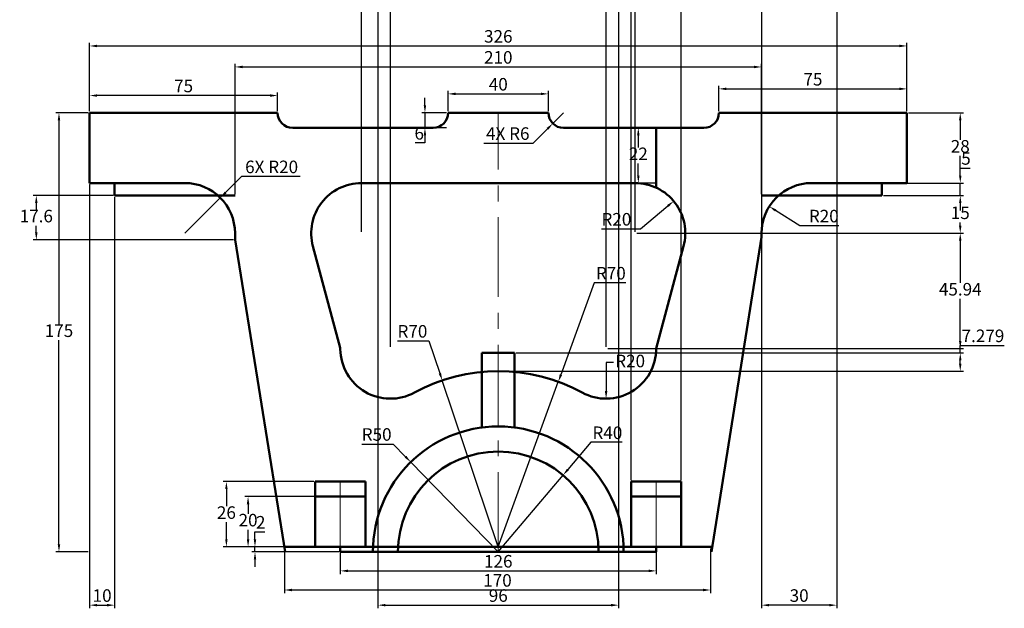
# Model space of a CAD drawing. Units: millimetres. Extents: x -44 to 350, y 28 to 429.
# Tile 1 of 2: x -43 to 350, y 28 to 262. Entities that reach past the tile are written whole.
import ezdxf

# ---------------------------------------------------------------- set-up
doc = ezdxf.new("R2010")
doc.units = ezdxf.units.MM
doc.linetypes.add('CENTER', pattern=[50.8, 31.75, -6.35, 6.35, -6.35])
for name, color, linetype, lineweight in [('M-CNTR', 1, 'CENTER', 18), ('M-DIMS', 2, 'Continuous', 25), ('M-OUTL', 7, 'Continuous', 50)]:
    doc.layers.add(name, color=color, linetype=linetype, lineweight=lineweight)
doc.styles.get("Standard").update_dxf_attribs({"font": 'arial.ttf'})
doc.dimstyles.new('ISO-25', dxfattribs={"dimtxt": 5, "dimasz": 3, "dimexe": 1.25, "dimexo": 0.625, "dimtad": 1, "dimtih": 1, "dimtoh": 1, "dimtxsty": 'Standard', "dimcen": 2.5, "dimadec": 0, "dimazin": 0, "dimtfac": 1, "dimtmove": 0, "dimatfit": 3, "dimfxl": 1, "dimarcsym": 0})

# ---------------------------------------------------------------- blocks, each defined once
blk = doc.blocks.new('*D1')
at = {"layer": 'Defpoints', "color": 0, "transparency": 16777216}
for p in [(310.7, 234.71), (235.7, 225.16), (310.7, 225.16)]:
    blk.add_point(p, dxfattribs=at)
at = {"layer": 'M-DIMS', "color": 0, "lineweight": -2, "transparency": 16777216}
for p, q in [((235.7, 225.78), (235.7, 235.96)), ((310.7, 225.78), (310.7, 235.96)), ((238.7, 234.71), (307.7, 234.71))]:
    blk.add_line(p, q, dxfattribs=at)
at = {"layer": 'M-DIMS', "color": 0, "transparency": 16777216}
for points in [[(238.7, 235.21), (238.7, 234.21), (235.7, 234.71)], [(307.7, 235.21), (307.7, 234.21), (310.7, 234.71)]]:
    blk.add_solid(points, dxfattribs=at)
at = {"layer": 'M-DIMS', "color": 0, "transparency": 16777216, "insert": (273.2, 237.88), "char_height": 5, "attachment_point": 5}
blk.add_mtext('75', dxfattribs=at)
blk = doc.blocks.new('*D2')
at = {"layer": 'Defpoints', "color": 0, "transparency": 16777216}
for p in [(167.7, 232.71), (127.7, 225.16), (167.7, 225.16)]:
    blk.add_point(p, dxfattribs=at)
at = {"layer": 'M-DIMS', "color": 0, "lineweight": -2, "transparency": 16777216}
for p, q in [((127.7, 225.78), (127.7, 233.96)), ((130.7, 232.71), (164.7, 232.71)), ((167.7, 225.78), (167.7, 233.96))]:
    blk.add_line(p, q, dxfattribs=at)
at = {"layer": 'M-DIMS', "color": 0, "transparency": 16777216}
for points in [[(130.7, 233.21), (130.7, 232.21), (127.7, 232.71)], [(164.7, 233.21), (164.7, 232.21), (167.7, 232.71)]]:
    blk.add_solid(points, dxfattribs=at)
at = {"layer": 'M-DIMS', "color": 0, "transparency": 16777216, "insert": (147.7, 235.89), "char_height": 5, "attachment_point": 5}
blk.add_mtext('40', dxfattribs=at)
blk = doc.blocks.new('*D3')
at = {"layer": 'Defpoints', "color": 0, "transparency": 16777216}
for p in [(-15.3, 232.04), (-15.3, 225.16), (59.7, 225.16)]:
    blk.add_point(p, dxfattribs=at)
at = {"layer": 'M-DIMS', "color": 0, "lineweight": -2, "transparency": 16777216}
for p, q in [((-15.3, 225.78), (-15.3, 233.29)), ((56.7, 232.04), (-12.3, 232.04)), ((59.7, 225.78), (59.7, 233.29))]:
    blk.add_line(p, q, dxfattribs=at)
at = {"layer": 'M-DIMS', "color": 0, "transparency": 16777216}
for points in [[(-12.3, 232.54), (-12.3, 231.54), (-15.3, 232.04)], [(56.7, 232.54), (56.7, 231.54), (59.7, 232.04)]]:
    blk.add_solid(points, dxfattribs=at)
at = {"layer": 'M-DIMS', "color": 0, "transparency": 16777216, "insert": (22.2, 235.21), "char_height": 5, "attachment_point": 5}
blk.add_mtext('75', dxfattribs=at)
blk = doc.blocks.new('*D4')
at = {"layer": 'Defpoints', "color": 0, "transparency": 16777216}
for p in [(252.7, 243.44), (42.7, 192.16), (252.7, 192.16)]:
    blk.add_point(p, dxfattribs=at)
at = {"layer": 'M-DIMS', "color": 0, "lineweight": -2, "transparency": 16777216}
for p, q in [((42.7, 192.78), (42.7, 244.69)), ((252.7, 192.78), (252.7, 244.69)), ((45.7, 243.44), (249.7, 243.44))]:
    blk.add_line(p, q, dxfattribs=at)
at = {"layer": 'M-DIMS', "color": 0, "transparency": 16777216}
for points in [[(45.7, 243.94), (45.7, 242.94), (42.7, 243.44)], [(249.7, 243.94), (249.7, 242.94), (252.7, 243.44)]]:
    blk.add_solid(points, dxfattribs=at)
at = {"layer": 'M-DIMS', "color": 0, "transparency": 16777216, "insert": (147.7, 246.62), "char_height": 5, "attachment_point": 5}
blk.add_mtext('210', dxfattribs=at)
blk = doc.blocks.new('*D5')
at = {"layer": 'Defpoints', "color": 0, "transparency": 16777216}
for p in [(310.7, 251.81), (-15.3, 225.16), (310.7, 225.16)]:
    blk.add_point(p, dxfattribs=at)
at = {"layer": 'M-DIMS', "color": 0, "lineweight": -2, "transparency": 16777216}
for p, q in [((-15.3, 225.78), (-15.3, 253.06)), ((-12.3, 251.81), (307.7, 251.81)), ((310.7, 225.78), (310.7, 253.06))]:
    blk.add_line(p, q, dxfattribs=at)
at = {"layer": 'M-DIMS', "color": 0, "transparency": 16777216}
for points in [[(-12.3, 252.31), (-12.3, 251.31), (-15.3, 251.81)], [(307.7, 252.31), (307.7, 251.31), (310.7, 251.81)]]:
    blk.add_solid(points, dxfattribs=at)
at = {"layer": 'M-DIMS', "color": 0, "transparency": 16777216, "insert": (147.7, 254.99), "char_height": 5, "attachment_point": 5}
blk.add_mtext('326', dxfattribs=at)
blk = doc.blocks.new('*D6')
at = {"layer": 'Defpoints', "color": 0, "transparency": 16777216}
for p in [(112.78, 85.95), (147.7, 50.16)]:
    blk.add_point(p, dxfattribs=at)
at = {"layer": 'M-DIMS', "color": 0, "lineweight": -2, "transparency": 16777216}
for p, q in [((93.22, 93.13), (105.78, 93.13)), ((105.78, 93.13), (110.69, 88.1)), ((147.7, 50.16), (112.78, 85.95))]:
    blk.add_line(p, q, dxfattribs=at)
at = {"layer": 'M-DIMS', "color": 0, "transparency": 16777216}
blk.add_solid([(111.05, 88.45), (110.33, 87.75), (112.78, 85.95)], dxfattribs=at)
at = {"layer": 'M-DIMS', "color": 0, "transparency": 16777216, "insert": (99.19, 96.31), "char_height": 5, "attachment_point": 5}
blk.add_mtext('R50', dxfattribs=at)
blk = doc.blocks.new('*D7')
at = {"layer": 'Defpoints', "color": 0, "transparency": 16777216}
for p in [(173.53, 80.7), (147.7, 50.16)]:
    blk.add_point(p, dxfattribs=at)
at = {"layer": 'M-DIMS', "color": 0, "lineweight": -2, "transparency": 16777216}
for p, q in [((184.62, 93.82), (175.46, 82.99)), ((197.17, 93.82), (184.62, 93.82)), ((147.7, 50.16), (173.53, 80.7))]:
    blk.add_line(p, q, dxfattribs=at)
at = {"layer": 'M-DIMS', "color": 0, "transparency": 16777216}
blk.add_solid([(175.08, 83.32), (175.85, 82.67), (173.53, 80.7)], dxfattribs=at)
at = {"layer": 'M-DIMS', "color": 0, "transparency": 16777216, "insert": (191.21, 96.99), "char_height": 5, "attachment_point": 5}
blk.add_mtext('R40', dxfattribs=at)
blk = doc.blocks.new('*D8')
at = {"layer": 'Defpoints', "color": 0, "transparency": 16777216}
for p in [(125.35, 118.5), (147.7, 52.16)]:
    blk.add_point(p, dxfattribs=at)
at = {"layer": 'M-DIMS', "color": 0, "lineweight": -2, "transparency": 16777216}
for p, q in [((107.5, 134.24), (120.05, 134.24)), ((120.05, 134.24), (124.4, 121.34)), ((147.7, 52.16), (125.35, 118.5))]:
    blk.add_line(p, q, dxfattribs=at)
at = {"layer": 'M-DIMS', "color": 0, "transparency": 16777216}
blk.add_solid([(124.87, 121.5), (123.92, 121.18), (125.35, 118.5)], dxfattribs=at)
at = {"layer": 'M-DIMS', "color": 0, "transparency": 16777216, "insert": (113.46, 137.42), "char_height": 5, "attachment_point": 5}
blk.add_mtext('R70', dxfattribs=at)
blk = doc.blocks.new('*D9')
at = {"layer": 'Defpoints', "color": 0, "transparency": 16777216}
for p in [(190.7, 131.22), (190.7, 111.22)]:
    blk.add_point(p, dxfattribs=at)
at = {"layer": 'M-DIMS', "color": 0, "lineweight": -2, "transparency": 16777216}
for p, q in [((193.7, 125.59), (190.7, 125.59)), ((190.7, 125.59), (190.7, 114.22))]:
    blk.add_line(p, q, dxfattribs=at)
at = {"layer": 'M-DIMS', "color": 0, "transparency": 16777216}
blk.add_solid([(190.2, 114.22), (191.2, 114.22), (190.7, 111.22)], dxfattribs=at)
at = {"layer": 'M-DIMS', "color": 0, "transparency": 16777216, "insert": (200.29, 125.59), "char_height": 5, "attachment_point": 5}
blk.add_mtext('R20', dxfattribs=at)
blk = doc.blocks.new('*D10')
at = {"layer": 'Defpoints', "color": 0, "transparency": 16777216}
for p in [(74.7, 78.16), (39.26, 52.16), (74.7, 52.16)]:
    blk.add_point(p, dxfattribs=at)
at = {"layer": 'M-DIMS', "color": 0, "lineweight": -2, "transparency": 16777216}
for p, q in [((74.08, 78.16), (38.01, 78.16)), ((39.26, 75.16), (39.26, 68.34)), ((39.26, 55.16), (39.26, 61.98)), ((74.08, 52.16), (38.01, 52.16))]:
    blk.add_line(p, q, dxfattribs=at)
at = {"layer": 'M-DIMS', "color": 0, "transparency": 16777216}
for points in [[(38.76, 75.16), (39.76, 75.16), (39.26, 78.16)], [(38.76, 55.16), (39.76, 55.16), (39.26, 52.16)]]:
    blk.add_solid(points, dxfattribs=at)
at = {"layer": 'M-DIMS', "color": 0, "transparency": 16777216, "insert": (39.26, 65.16), "char_height": 5, "attachment_point": 5}
blk.add_mtext('26', dxfattribs=at)
blk = doc.blocks.new('*D11')
at = {"layer": 'Defpoints', "color": 0, "transparency": 16777216}
for p in [(74.7, 72.16), (47.91, 52.16), (74.7, 52.16)]:
    blk.add_point(p, dxfattribs=at)
at = {"layer": 'M-DIMS', "color": 0, "lineweight": -2, "transparency": 16777216}
for p, q in [((74.08, 72.16), (46.66, 72.16)), ((47.91, 69.16), (47.91, 65.34)), ((47.91, 55.16), (47.91, 58.98)), ((74.08, 52.16), (46.66, 52.16))]:
    blk.add_line(p, q, dxfattribs=at)
at = {"layer": 'M-DIMS', "color": 0, "transparency": 16777216}
for points in [[(47.41, 69.16), (48.41, 69.16), (47.91, 72.16)], [(47.41, 55.16), (48.41, 55.16), (47.91, 52.16)]]:
    blk.add_solid(points, dxfattribs=at)
at = {"layer": 'M-DIMS', "color": 0, "transparency": 16777216, "insert": (47.91, 62.16), "char_height": 5, "attachment_point": 5}
blk.add_mtext('20', dxfattribs=at)
blk = doc.blocks.new('*D12')
at = {"layer": 'Defpoints', "color": 0, "transparency": 16777216}
for p in [(50.67, 52.16), (84.7, 52.16), (84.7, 50.16)]:
    blk.add_point(p, dxfattribs=at)
at = {"layer": 'M-DIMS', "color": 0, "lineweight": -2, "transparency": 16777216}
for p, q in [((50.67, 55.16), (50.67, 58.16)), ((50.67, 58.16), (54.61, 58.16)), ((84.08, 52.16), (49.42, 52.16)), ((50.67, 50.16), (50.67, 52.16)), ((84.08, 50.16), (49.42, 50.16)), ((50.67, 47.16), (50.67, 44.16))]:
    blk.add_line(p, q, dxfattribs=at)
at = {"layer": 'M-DIMS', "color": 0, "transparency": 16777216}
for points in [[(50.17, 55.16), (51.17, 55.16), (50.67, 52.16)], [(50.17, 47.16), (51.17, 47.16), (50.67, 50.16)]]:
    blk.add_solid(points, dxfattribs=at)
at = {"layer": 'M-DIMS', "color": 0, "transparency": 16777216, "insert": (52.95, 61.3), "char_height": 5, "attachment_point": 5}
blk.add_mtext('2', dxfattribs=at)
blk = doc.blocks.new('*D13')
at = {"layer": 'Defpoints', "color": 0, "transparency": 16777216}
for p in [(84.7, 52.16), (210.7, 52.16), (210.7, 42.57)]:
    blk.add_point(p, dxfattribs=at)
at = {"layer": 'M-DIMS', "color": 0, "lineweight": -2, "transparency": 16777216}
for p, q in [((84.7, 51.53), (84.7, 41.32)), ((210.7, 51.53), (210.7, 41.32)), ((87.7, 42.57), (207.7, 42.57))]:
    blk.add_line(p, q, dxfattribs=at)
at = {"layer": 'M-DIMS', "color": 0, "transparency": 16777216}
for points in [[(87.7, 43.07), (87.7, 42.07), (84.7, 42.57)], [(207.7, 43.07), (207.7, 42.07), (210.7, 42.57)]]:
    blk.add_solid(points, dxfattribs=at)
at = {"layer": 'M-DIMS', "color": 0, "transparency": 16777216, "insert": (147.7, 45.75), "char_height": 5, "attachment_point": 5}
blk.add_mtext('126', dxfattribs=at)
blk = doc.blocks.new('*D14')
at = {"layer": 'Defpoints', "color": 0, "transparency": 16777216}
for p in [(62.38, 52.16), (232.38, 52.16), (232.38, 34.96)]:
    blk.add_point(p, dxfattribs=at)
at = {"layer": 'M-DIMS', "color": 0, "lineweight": -2, "transparency": 16777216}
for p, q in [((62.38, 51.53), (62.38, 33.71)), ((232.38, 51.53), (232.38, 33.71)), ((65.38, 34.96), (229.38, 34.96))]:
    blk.add_line(p, q, dxfattribs=at)
at = {"layer": 'M-DIMS', "color": 0, "transparency": 16777216}
for points in [[(65.38, 35.46), (65.38, 34.46), (62.38, 34.96)], [(229.38, 35.46), (229.38, 34.46), (232.38, 34.96)]]:
    blk.add_solid(points, dxfattribs=at)
at = {"layer": 'M-DIMS', "color": 0, "transparency": 16777216, "insert": (147.38, 38.14), "char_height": 5, "attachment_point": 5}
blk.add_mtext('170', dxfattribs=at)
blk = doc.blocks.new('*D15')
at = {"layer": 'Defpoints', "color": 0, "transparency": 16777216}
for p in [(-15.3, 225.16), (-27.51, 50.16), (-15.3, 50.16)]:
    blk.add_point(p, dxfattribs=at)
at = {"layer": 'M-DIMS', "color": 0, "lineweight": -2, "transparency": 16777216}
for p, q in [((-15.92, 225.16), (-28.76, 225.16)), ((-27.51, 222.16), (-27.51, 140.84)), ((-27.51, 53.16), (-27.51, 134.48)), ((-15.92, 50.16), (-28.76, 50.16))]:
    blk.add_line(p, q, dxfattribs=at)
at = {"layer": 'M-DIMS', "color": 0, "transparency": 16777216}
for points in [[(-28.01, 222.16), (-27.01, 222.16), (-27.51, 225.16)], [(-28.01, 53.16), (-27.01, 53.16), (-27.51, 50.16)]]:
    blk.add_solid(points, dxfattribs=at)
at = {"layer": 'M-DIMS', "color": 0, "transparency": 16777216, "insert": (-27.51, 137.66), "char_height": 5, "attachment_point": 5}
blk.add_mtext('175', dxfattribs=at)
blk = doc.blocks.new('*D16')
at = {"layer": 'Defpoints', "color": 0, "transparency": 16777216}
for p in [(217.66, 189.97), (202.3, 177.16)]:
    blk.add_point(p, dxfattribs=at)
at = {"layer": 'M-DIMS', "color": 0, "lineweight": -2, "transparency": 16777216}
for p, q in [((204.39, 178.9), (215.36, 188.05)), ((188.83, 178.9), (204.39, 178.9))]:
    blk.add_line(p, q, dxfattribs=at)
at = {"layer": 'M-DIMS', "color": 0, "transparency": 16777216}
blk.add_solid([(215.03, 188.44), (215.68, 187.67), (217.66, 189.97)], dxfattribs=at)
at = {"layer": 'M-DIMS', "color": 0, "transparency": 16777216, "insert": (194.8, 182.08), "char_height": 5, "attachment_point": 5}
blk.add_mtext('R20', dxfattribs=at)
blk = doc.blocks.new('*D17')
at = {"layer": 'Defpoints', "color": 0, "transparency": 16777216}
for p in [(255.78, 187.83), (272.7, 177.16)]:
    blk.add_point(p, dxfattribs=at)
at = {"layer": 'M-DIMS', "color": 0, "lineweight": -2, "transparency": 16777216}
for p, q in [((267.93, 180.17), (258.32, 186.23)), ((283.49, 180.17), (267.93, 180.17))]:
    blk.add_line(p, q, dxfattribs=at)
at = {"layer": 'M-DIMS', "color": 0, "transparency": 16777216}
blk.add_solid([(258.59, 186.65), (258.05, 185.81), (255.78, 187.83)], dxfattribs=at)
at = {"layer": 'M-DIMS', "color": 0, "transparency": 16777216, "insert": (277.52, 183.35), "char_height": 5, "attachment_point": 5}
blk.add_mtext('R20', dxfattribs=at)
blk = doc.blocks.new('*D18')
at = {"layer": 'Defpoints', "color": 0, "transparency": 16777216}
for p in [(210.7, 219.16), (203.55, 197.16), (210.7, 197.16)]:
    blk.add_point(p, dxfattribs=at)
at = {"layer": 'M-DIMS', "color": 0, "lineweight": -2, "transparency": 16777216}
for p, q in [((210.08, 219.16), (202.3, 219.16)), ((203.55, 216.16), (203.55, 211.3)), ((203.55, 200.16), (203.55, 205.02)), ((210.08, 197.16), (202.3, 197.16))]:
    blk.add_line(p, q, dxfattribs=at)
at = {"layer": 'M-DIMS', "color": 0, "transparency": 16777216}
for points in [[(203.05, 216.16), (204.05, 216.16), (203.55, 219.16)], [(203.05, 200.16), (204.05, 200.16), (203.55, 197.16)]]:
    blk.add_solid(points, dxfattribs=at)
at = {"layer": 'M-DIMS', "color": 0, "transparency": 16777216, "insert": (203.55, 208.16), "char_height": 5, "attachment_point": 5}
blk.add_mtext('22', dxfattribs=at)
blk = doc.blocks.new('*D19')
at = {"layer": 'Defpoints', "color": 0, "transparency": 16777216}
for p in [(127.7, 225.16), (118.45, 219.16), (127.7, 219.16)]:
    blk.add_point(p, dxfattribs=at)
at = {"layer": 'M-DIMS', "color": 0, "lineweight": -2, "transparency": 16777216}
for p, q in [((118.45, 228.16), (118.45, 231.16)), ((127.08, 225.16), (117.2, 225.16)), ((118.45, 225.16), (118.45, 219.16)), ((127.08, 219.16), (117.2, 219.16)), ((118.45, 216.16), (118.45, 213.16)), ((118.45, 213.16), (114.52, 213.16))]:
    blk.add_line(p, q, dxfattribs=at)
at = {"layer": 'M-DIMS', "color": 0, "transparency": 16777216}
for points in [[(117.95, 228.16), (118.95, 228.16), (118.45, 225.16)], [(117.95, 216.16), (118.95, 216.16), (118.45, 219.16)]]:
    blk.add_solid(points, dxfattribs=at)
at = {"layer": 'M-DIMS', "color": 0, "transparency": 16777216, "insert": (116.17, 216.34), "char_height": 5, "attachment_point": 5}
blk.add_mtext('6', dxfattribs=at)
blk = doc.blocks.new('*D30')
at = {"layer": 'Defpoints', "color": 0, "transparency": 16777216}
for p in [(99.7, 292.57), (195.7, 292.57), (195.7, 28.91)]:
    blk.add_point(p, dxfattribs=at)
at = {"layer": 'M-DIMS', "color": 0, "lineweight": -2, "transparency": 16777216}
for p, q in [((99.7, 291.94), (99.7, 27.66)), ((195.7, 291.94), (195.7, 27.66)), ((102.7, 28.91), (192.7, 28.91))]:
    blk.add_line(p, q, dxfattribs=at)
at = {"layer": 'M-DIMS', "color": 0, "transparency": 16777216}
for points in [[(102.7, 29.41), (102.7, 28.41), (99.7, 28.91)], [(192.7, 29.41), (192.7, 28.41), (195.7, 28.91)]]:
    blk.add_solid(points, dxfattribs=at)
at = {"layer": 'M-DIMS', "color": 0, "transparency": 16777216, "insert": (147.7, 32.09), "char_height": 5, "attachment_point": 5}
blk.add_mtext('96', dxfattribs=at)
blk = doc.blocks.new('*D31')
at = {"layer": 'Defpoints', "color": 0, "transparency": 16777216}
for p in [(282.7, 339.57), (252.7, 319.57), (252.7, 28.91)]:
    blk.add_point(p, dxfattribs=at)
at = {"layer": 'M-DIMS', "color": 0, "lineweight": -2, "transparency": 16777216}
for p, q in [((282.7, 338.94), (282.7, 27.66)), ((252.7, 318.94), (252.7, 27.66)), ((279.7, 28.91), (255.7, 28.91))]:
    blk.add_line(p, q, dxfattribs=at)
at = {"layer": 'M-DIMS', "color": 0, "transparency": 16777216}
for points in [[(255.7, 29.41), (255.7, 28.41), (252.7, 28.91)], [(279.7, 29.41), (279.7, 28.41), (282.7, 28.91)]]:
    blk.add_solid(points, dxfattribs=at)
at = {"layer": 'M-DIMS', "color": 0, "transparency": 16777216, "insert": (267.7, 32.09), "char_height": 5, "attachment_point": 5}
blk.add_mtext('30', dxfattribs=at)
blk = doc.blocks.new('*D33')
at = {"layer": 'Defpoints', "color": 0, "transparency": 16777216}
for p in [(310.7, 225.16), (331.95, 225.16), (310.7, 197.16)]:
    blk.add_point(p, dxfattribs=at)
at = {"layer": 'M-DIMS', "color": 0, "lineweight": -2, "transparency": 16777216}
for p, q in [((311.33, 225.16), (333.2, 225.16)), ((331.95, 222.16), (331.95, 214.34)), ((331.95, 200.16), (331.95, 207.98)), ((311.33, 197.16), (333.2, 197.16))]:
    blk.add_line(p, q, dxfattribs=at)
at = {"layer": 'M-DIMS', "color": 0, "transparency": 16777216}
for points in [[(331.45, 222.16), (332.45, 222.16), (331.95, 225.16)], [(331.45, 200.16), (332.45, 200.16), (331.95, 197.16)]]:
    blk.add_solid(points, dxfattribs=at)
at = {"layer": 'M-DIMS', "color": 0, "transparency": 16777216, "insert": (331.95, 211.16), "char_height": 5, "attachment_point": 5}
blk.add_mtext('28', dxfattribs=at)
blk = doc.blocks.new('*D34')
at = {"layer": 'Defpoints', "color": 0, "transparency": 16777216}
for p in [(300.7, 197.16), (331.95, 197.16), (300.7, 192.16)]:
    blk.add_point(p, dxfattribs=at)
at = {"layer": 'M-DIMS', "color": 0, "lineweight": -2, "transparency": 16777216}
for p, q in [((331.95, 200.16), (331.95, 203.16)), ((331.95, 203.16), (335.89, 203.16)), ((301.33, 197.16), (333.2, 197.16)), ((331.95, 192.16), (331.95, 197.16)), ((301.33, 192.16), (333.2, 192.16)), ((331.95, 189.16), (331.95, 186.16))]:
    blk.add_line(p, q, dxfattribs=at)
at = {"layer": 'M-DIMS', "color": 0, "transparency": 16777216}
for points in [[(331.45, 200.16), (332.45, 200.16), (331.95, 197.16)], [(331.45, 189.16), (332.45, 189.16), (331.95, 192.16)]]:
    blk.add_solid(points, dxfattribs=at)
at = {"layer": 'M-DIMS', "color": 0, "transparency": 16777216, "insert": (334.23, 206.33), "char_height": 5, "attachment_point": 5}
blk.add_mtext('5', dxfattribs=at)
blk = doc.blocks.new('*D35')
at = {"layer": 'Defpoints', "color": 0, "transparency": 16777216}
for p in [(-15.3, 197.16), (-5.3, 192.16), (-5.3, 28.91)]:
    blk.add_point(p, dxfattribs=at)
at = {"layer": 'M-DIMS', "color": 0, "lineweight": -2, "transparency": 16777216}
for p, q in [((-15.3, 196.53), (-15.3, 27.66)), ((-5.3, 191.53), (-5.3, 27.66)), ((-12.3, 28.91), (-8.3, 28.91))]:
    blk.add_line(p, q, dxfattribs=at)
at = {"layer": 'M-DIMS', "color": 0, "transparency": 16777216}
for points in [[(-12.3, 29.41), (-12.3, 28.41), (-15.3, 28.91)], [(-8.3, 29.41), (-8.3, 28.41), (-5.3, 28.91)]]:
    blk.add_solid(points, dxfattribs=at)
at = {"layer": 'M-DIMS', "color": 0, "transparency": 16777216, "insert": (-10.3, 32.09), "char_height": 5, "attachment_point": 5}
blk.add_mtext('10', dxfattribs=at)
blk = doc.blocks.new('*D36')
at = {"layer": 'Defpoints', "color": 0, "transparency": 16777216}
for p in [(202.3, 407.82), (93.1, 177.16), (202.3, 177.16)]:
    blk.add_point(p, dxfattribs=at)
at = {"layer": 'M-DIMS', "color": 0, "lineweight": -2, "transparency": 16777216}
for p, q in [((93.1, 177.78), (93.1, 409.07)), ((202.3, 177.78), (202.3, 409.07)), ((96.1, 407.82), (199.3, 407.82))]:
    blk.add_line(p, q, dxfattribs=at)
at = {"layer": 'M-DIMS', "color": 0, "transparency": 16777216}
for points in [[(96.1, 408.32), (96.1, 407.32), (93.1, 407.82)], [(199.3, 408.32), (199.3, 407.32), (202.3, 407.82)]]:
    blk.add_solid(points, dxfattribs=at)
at = {"layer": 'M-DIMS', "color": 0, "transparency": 16777216, "insert": (147.7, 411), "char_height": 5, "attachment_point": 5}
blk.add_mtext('109.2', dxfattribs=at)
blk = doc.blocks.new('*D37')
at = {"layer": 'Defpoints', "color": 0, "transparency": 16777216}
for p in [(190.7, 407.82), (104.7, 131.22), (190.7, 131.22)]:
    blk.add_point(p, dxfattribs=at)
at = {"layer": 'M-DIMS', "color": 0, "lineweight": -2, "transparency": 16777216}
for p, q in [((104.7, 131.85), (104.7, 409.07)), ((190.7, 131.85), (190.7, 409.07)), ((107.7, 407.82), (187.7, 407.82))]:
    blk.add_line(p, q, dxfattribs=at)
at = {"layer": 'M-DIMS', "color": 0, "transparency": 16777216}
for points in [[(107.7, 408.32), (107.7, 407.32), (104.7, 407.82)], [(187.7, 408.32), (187.7, 407.32), (190.7, 407.82)]]:
    blk.add_solid(points, dxfattribs=at)
at = {"layer": 'M-DIMS', "color": 0, "transparency": 16777216, "insert": (147.7, 411), "char_height": 5, "attachment_point": 5}
blk.add_mtext('86', dxfattribs=at)
blk = doc.blocks.new('*D38')
at = {"layer": 'Defpoints', "color": 0, "transparency": 16777216}
for p in [(154.2, 129.44), (331.95, 129.44), (147.7, 122.16)]:
    blk.add_point(p, dxfattribs=at)
at = {"layer": 'M-DIMS', "color": 0, "lineweight": -2, "transparency": 16777216}
for p, q in [((331.95, 129.44), (331.95, 132.44)), ((331.95, 132.44), (349.42, 132.44)), ((154.83, 129.44), (333.2, 129.44)), ((331.95, 125.16), (331.95, 126.44)), ((148.33, 122.16), (333.2, 122.16))]:
    blk.add_line(p, q, dxfattribs=at)
at = {"layer": 'M-DIMS', "color": 0, "transparency": 16777216}
for points in [[(331.45, 126.44), (332.45, 126.44), (331.95, 129.44)], [(331.45, 125.16), (332.45, 125.16), (331.95, 122.16)]]:
    blk.add_solid(points, dxfattribs=at)
at = {"layer": 'M-DIMS', "color": 0, "transparency": 16777216, "insert": (341, 135.62), "char_height": 5, "attachment_point": 5}
blk.add_mtext('7.279', dxfattribs=at)
blk = doc.blocks.new('*D39')
at = {"layer": 'Defpoints', "color": 0, "transparency": 16777216}
for p in [(202.3, 177.16), (331.95, 177.16), (190.7, 131.22)]:
    blk.add_point(p, dxfattribs=at)
at = {"layer": 'M-DIMS', "color": 0, "lineweight": -2, "transparency": 16777216}
for p, q in [((202.93, 177.16), (333.2, 177.16)), ((331.95, 174.16), (331.95, 157.37)), ((331.95, 134.22), (331.95, 151.01)), ((191.33, 131.22), (333.2, 131.22))]:
    blk.add_line(p, q, dxfattribs=at)
at = {"layer": 'M-DIMS', "color": 0, "transparency": 16777216}
for points in [[(331.45, 174.16), (332.45, 174.16), (331.95, 177.16)], [(331.45, 134.22), (332.45, 134.22), (331.95, 131.22)]]:
    blk.add_solid(points, dxfattribs=at)
at = {"layer": 'M-DIMS', "color": 0, "transparency": 16777216, "insert": (331.95, 154.19), "char_height": 5, "attachment_point": 5}
blk.add_mtext('45.94', dxfattribs=at)
blk = doc.blocks.new('*D40')
at = {"layer": 'Defpoints', "color": 0, "transparency": 16777216}
for p in [(300.7, 192.16), (331.95, 192.16), (202.3, 177.16)]:
    blk.add_point(p, dxfattribs=at)
at = {"layer": 'M-DIMS', "color": 0, "lineweight": -2, "transparency": 16777216}
for p, q in [((301.33, 192.16), (333.2, 192.16)), ((331.95, 189.16), (331.95, 187.84)), ((331.95, 180.16), (331.95, 181.48)), ((202.93, 177.16), (333.2, 177.16))]:
    blk.add_line(p, q, dxfattribs=at)
at = {"layer": 'M-DIMS', "color": 0, "transparency": 16777216}
for points in [[(331.45, 189.16), (332.45, 189.16), (331.95, 192.16)], [(331.45, 180.16), (332.45, 180.16), (331.95, 177.16)]]:
    blk.add_solid(points, dxfattribs=at)
at = {"layer": 'M-DIMS', "color": 0, "transparency": 16777216, "insert": (331.95, 184.66), "char_height": 5, "attachment_point": 5}
blk.add_mtext('15', dxfattribs=at)
blk = doc.blocks.new('*D41')
at = {"layer": 'Defpoints', "color": 0, "transparency": 16777216}
for p in [(-36.55, 192.16), (-5.3, 192.16), (42.7, 174.56)]:
    blk.add_point(p, dxfattribs=at)
at = {"layer": 'M-DIMS', "color": 0, "lineweight": -2, "transparency": 16777216}
for p, q in [((-5.92, 192.16), (-37.8, 192.16)), ((-36.55, 189.16), (-36.55, 186.54)), ((-36.55, 177.56), (-36.55, 180.18)), ((42.08, 174.56), (-37.8, 174.56))]:
    blk.add_line(p, q, dxfattribs=at)
at = {"layer": 'M-DIMS', "color": 0, "transparency": 16777216}
for points in [[(-37.05, 189.16), (-36.05, 189.16), (-36.55, 192.16)], [(-37.05, 177.56), (-36.05, 177.56), (-36.55, 174.56)]]:
    blk.add_solid(points, dxfattribs=at)
at = {"layer": 'M-DIMS', "color": 0, "transparency": 16777216, "insert": (-36.55, 183.36), "char_height": 5, "attachment_point": 5}
blk.add_mtext('17.6', dxfattribs=at)
blk = doc.blocks.new('*D42')
at = {"layer": 'Defpoints', "color": 0, "transparency": 16777216}
for p in [(220.7, 407.82), (200.7, 78.16), (220.7, 78.16)]:
    blk.add_point(p, dxfattribs=at)
at = {"layer": 'M-DIMS', "color": 0, "lineweight": -2, "transparency": 16777216}
for p, q in [((200.7, 78.78), (200.7, 409.07)), ((220.7, 78.78), (220.7, 409.07)), ((203.7, 407.82), (217.7, 407.82))]:
    blk.add_line(p, q, dxfattribs=at)
at = {"layer": 'M-DIMS', "color": 0, "transparency": 16777216}
for points in [[(203.7, 408.32), (203.7, 407.32), (200.7, 407.82)], [(217.7, 408.32), (217.7, 407.32), (220.7, 407.82)]]:
    blk.add_solid(points, dxfattribs=at)
at = {"layer": 'M-DIMS', "color": 0, "transparency": 16777216, "insert": (210.7, 411), "char_height": 5, "attachment_point": 5}
blk.add_mtext('20', dxfattribs=at)
blk = doc.blocks.new('*D49')
at = {"layer": 'Defpoints', "color": 0, "transparency": 16777216}
for p in [(36.84, 191.3), (22.7, 177.16)]:
    blk.add_point(p, dxfattribs=at)
at = {"layer": 'M-DIMS', "color": 0, "lineweight": -2, "transparency": 16777216}
for p, q in [((45.33, 199.79), (38.96, 193.42)), ((68.65, 199.79), (45.33, 199.79)), ((22.7, 177.16), (36.84, 191.3))]:
    blk.add_line(p, q, dxfattribs=at)
at = {"layer": 'M-DIMS', "color": 0, "transparency": 16777216}
blk.add_solid([(38.61, 193.78), (39.32, 193.07), (36.84, 191.3)], dxfattribs=at)
at = {"layer": 'M-DIMS', "color": 0, "transparency": 16777216, "insert": (57.3, 202.96), "char_height": 5, "attachment_point": 5}
blk.add_mtext('6X R20', dxfattribs=at)
blk = doc.blocks.new('*D50')
at = {"layer": 'Defpoints', "color": 0, "transparency": 16777216}
for p in [(171.64, 117.94), (147.7, 52.16)]:
    blk.add_point(p, dxfattribs=at)
at = {"layer": 'M-DIMS', "color": 0, "lineweight": -2, "transparency": 16777216}
for p, q in [((186, 157.41), (172.67, 120.76)), ((198.56, 157.41), (186, 157.41)), ((147.7, 52.16), (171.64, 117.94))]:
    blk.add_line(p, q, dxfattribs=at)
at = {"layer": 'M-DIMS', "color": 0, "transparency": 16777216}
blk.add_solid([(172.2, 120.93), (173.14, 120.59), (171.64, 117.94)], dxfattribs=at)
at = {"layer": 'M-DIMS', "color": 0, "transparency": 16777216, "insert": (192.59, 160.58), "char_height": 5, "attachment_point": 5}
blk.add_mtext('R70', dxfattribs=at)
blk = doc.blocks.new('*D51')
at = {"layer": 'Defpoints', "color": 0, "transparency": 16777216}
for p in [(173.7, 225.16), (169.46, 220.92)]:
    blk.add_point(p, dxfattribs=at)
at = {"layer": 'M-DIMS', "color": 0, "lineweight": -2, "transparency": 16777216}
for p, q in [((173.7, 225.16), (169.46, 220.92)), ((161.61, 213.06), (167.34, 218.8)), ((141.98, 213.06), (161.61, 213.06))]:
    blk.add_line(p, q, dxfattribs=at)
at = {"layer": 'M-DIMS', "color": 0, "transparency": 16777216}
blk.add_solid([(166.98, 219.15), (167.69, 218.44), (169.46, 220.92)], dxfattribs=at)
at = {"layer": 'M-DIMS', "color": 0, "transparency": 16777216, "insert": (151.48, 216.24), "char_height": 5, "attachment_point": 5}
blk.add_mtext('4X R6', dxfattribs=at)

msp = doc.modelspace()

# ---------------------------------------------------------------- linework, layer by layer
at = {"layer": 'M-CNTR'}
for p, q in [((147.7005, 50.1598), (147.7005, 225.1598)), ((147.7005, 100.1598), (147.7005, 129.4388)), ((84.7005, 52.1598), (84.7005, 78.1598)), ((210.7005, 52.1598), (210.7005, 78.1598)), ((84.7005, 52.1598), (84.7005, 72.1598)), ((147.7005, 50.1598), (147.7005, 58.3693)), ((147.7005, 50.1598), (147.7005, 52.1598))]:
    msp.add_line(p, q, dxfattribs=at)
at = {"layer": 'M-OUTL'}
for p, q in [((59.7005, 225.1598), (-15.2995, 225.1598)), ((-15.2995, 225.1598), (-15.2995, 197.1598)), ((59.7005, 225.1598), (59.7005, 225.1598)), ((147.7005, 225.1598), (127.7005, 225.1598)), ((127.7005, 225.1598), (127.7005, 225.1598)), ((147.7005, 225.1598), (127.7005, 225.1598)), ((147.7005, 225.1598), (167.7005, 225.1598)), ((147.7005, 225.1598), (167.7005, 225.1598)), ((167.7005, 225.1598), (167.7005, 225.1598)), ((235.7005, 225.1598), (235.7005, 225.1598)), ((235.7005, 225.1598), (310.7005, 225.1598)), ((310.7005, 225.1598), (310.7005, 197.1598)), ((65.7005, 219.1598), (118.8026, 219.1598)), ((121.7005, 219.1598), (118.8026, 219.1598)), ((173.7005, 219.1598), (184.4392, 219.1598)), ((184.4392, 219.1598), (191.152, 219.1598)), ((229.7005, 219.1598), (191.152, 219.1598)), ((210.7005, 195.3118), (210.7005, 219.1598)), ((210.7005, 219.1598), (210.7005, 197.1598)), ((-15.2995, 197.1598), (22.7005, 197.1598)), ((-15.2995, 197.1598), (-5.2995, 197.1598)), ((-5.2995, 197.1598), (-5.2995, 192.1598)), ((202.3037, 197.1598), (93.0974, 197.1598)), ((310.7005, 197.1598), (272.7005, 197.1598)), ((310.7005, 197.1598), (300.7005, 197.1598)), ((300.7005, 197.1598), (300.7005, 192.1598)), ((-5.2995, 192.1598), (42.7005, 192.1598)), ((300.7005, 192.1598), (252.7005, 192.1598)), ((42.7005, 177.1598), (42.7005, 174.5602)), ((252.7005, 177.1598), (252.7005, 175.5915)), ((42.7005, 174.5602), (62.7005, 50.1598)), ((252.7005, 175.5915), (232.7005, 50.1598)), ((84.634, 131.4713), (73.7788, 171.9835)), ((210.7005, 131.2231), (221.6222, 171.9835)), ((147.7005, 129.4388), (141.2005, 129.4388)), ((141.2005, 129.4388), (141.2005, 99.7355)), ((147.7005, 129.4388), (154.2005, 129.4388)), ((154.2005, 129.4388), (154.2005, 99.7355)), ((84.7005, 78.1598), (74.7005, 78.1598)), ((74.7005, 78.1598), (74.7005, 72.1598)), ((84.7005, 78.1598), (94.7005, 78.1598)), ((94.7005, 78.1598), (94.7005, 70.2284)), ((210.7005, 78.1598), (200.7005, 78.1598)), ((200.7005, 78.1598), (200.7005, 72.1598)), ((210.7005, 78.1598), (220.7005, 78.1598)), ((220.7005, 78.1598), (220.7005, 70.2284)), ((84.7005, 72.1598), (74.7005, 72.1598)), ((74.7005, 72.1598), (74.7005, 52.1598)), ((84.7005, 72.1598), (94.7005, 72.1598)), ((94.7005, 72.1598), (94.7005, 52.1598)), ((210.7005, 72.1598), (200.7005, 72.1598)), ((200.7005, 72.1598), (200.7005, 52.1598)), ((210.7005, 72.1598), (220.7005, 72.1598)), ((220.7005, 72.1598), (220.7005, 52.1598)), ((147.7005, 52.1598), (62.379, 52.1598)), ((84.7005, 50.1598), (84.7005, 52.1598)), ((147.7005, 52.1598), (233.0194, 52.1598)), ((210.7005, 50.1598), (210.7005, 52.1598)), ((84.7005, 50.1598), (210.7005, 50.1598)), ((97.7005, 50.1598), (147.7005, 50.1598)), ((147.7005, 50.1598), (97.7005, 50.1598)), ((147.7005, 50.1598), (197.7005, 50.1598))]:
    msp.add_line(p, q, dxfattribs=at)
for centre, radius, start, end in [((65.7005, 225.1598), 6, 180, 270), ((121.7005, 225.1598), 6, 270, 0), ((173.7005, 225.1598), 6, 180, 270), ((229.7005, 225.1598), 6, 270, 0), ((22.7005, 177.1598), 20, 0, 90), ((93.0974, 177.1598), 20, 90, 195), ((202.3037, 177.1598), 20, 345, 90), ((272.7005, 177.1598), 20, 90, 180), ((82.7022, 130.9536), 2, 0.701797, 15), ((104.7005, 131.2231), 20, 180.701797, 298.540365), ((190.7005, 131.2231), 20, 241.459635, 0), ((147.7005, 52.1598), 70, 61.459635, 118.540365), ((147.7005, 50.1598), 50, 0, 180), ((147.7005, 50.1598), 40, 0, 180)]:
    msp.add_arc(centre, radius, start, end, dxfattribs=at)

# ---------------------------------------------------------------- dimensions: what is measured, and where the dimension line sits
at = {"layer": 'M-DIMS'}
for base, p1, p2, override, picture, middle in [((202.3037, 407.8182), (93.0974, 177.1598), (202.3037, 177.1598), {"dimdec": 1, "dimlfac": 1, "dimrnd": 0, "dimzin": 0, "dimdsep": 46, "dimlunit": 2}, '*D36', (147.7005, 410.9961)), ((190.7005, 407.8182), (104.7005, 131.2231), (190.7005, 131.2231), {"dimdec": 0, "dimlfac": 1, "dimrnd": 0, "dimzin": 0, "dimdsep": 46, "dimlunit": 2}, '*D37', (147.7005, 410.9961)), ((220.7005, 407.8182), (200.7005, 78.1598), (220.7005, 78.1598), {"dimdec": 0, "dimlfac": 1, "dimrnd": 0, "dimzin": 0, "dimdsep": 46, "dimlunit": 2}, '*D42', (210.7005, 410.9961)), ((252.7005, 28.9098), (282.7005, 339.5682), (252.7005, 319.5682), {"dimdec": 0, "dimlfac": 1, "dimrnd": 0, "dimzin": 0, "dimdsep": 46, "dimlunit": 2}, '*D31', (267.7005, 32.0894)), ((195.7005, 28.9098), (99.7005, 292.5682), (195.7005, 292.5682), {"dimdec": 0, "dimlfac": 1, "dimrnd": 0, "dimzin": 0, "dimdsep": 46, "dimlunit": 2}, '*D30', (147.7005, 32.0877)), ((310.7005, 251.8083), (-15.2995, 225.1598), (310.7005, 225.1598), {"dimclrd": 0, "dimclre": 0, "dimclrt": 0}, '*D5', (147.7005, 254.9879)), ((252.7005, 243.4406), (42.7005, 192.1598), (252.7005, 192.1598), {"dimclrd": 0, "dimclre": 0, "dimclrt": 0}, '*D4', (147.7005, 246.6185)), ((310.7005, 234.715), (235.7005, 225.1598), (310.7005, 225.1598), {"dimclrd": 0, "dimclre": 0, "dimclrt": 0}, '*D1', (273.2005, 237.8826)), ((-15.2995, 232.042), (59.7005, 225.1598), (-15.2995, 225.1598), {"dimclrd": 0, "dimclre": 0, "dimclrt": 0}, '*D3', (22.2005, 235.2096)), ((167.7005, 232.7125), (127.7005, 225.1598), (167.7005, 225.1598), {"dimclrd": 0, "dimclre": 0, "dimclrt": 0}, '*D2', (147.7005, 235.8903)), ((-5.2995, 28.9098), (-15.2995, 197.1598), (-5.2995, 192.1598), {"dimdec": 0, "dimlfac": 1, "dimrnd": 0, "dimzin": 0, "dimdsep": 46, "dimlunit": 2}, '*D35', (-10.2995, 32.0877)), ((232.379, 34.9611), (62.379, 52.1598), (232.379, 52.1598), {"dimclrd": 0, "dimclre": 0, "dimclrt": 0}, '*D14', (147.379, 38.1389)), ((210.7005, 42.5734), (84.7005, 52.1598), (210.7005, 52.1598), {"dimclrd": 0, "dimclre": 0, "dimclrt": 0}, '*D13', (147.7005, 45.7513))]:
    dim = msp.add_linear_dim(base=base, p1=p1, p2=p2, dimstyle='ISO-25', override=override, dxfattribs=at)
    dim.commit()
    dim.dimension.update_dxf_attribs({"geometry": picture, "text_midpoint": middle})
for base, p1, p2, override, picture, middle in [((118.4493, 219.1598), (127.7005, 225.1598), (127.7005, 219.1598), {"dimclrd": 0, "dimclre": 0, "dimclrt": 0}, '*D19', (116.1735, 216.3377)), ((-27.5061, 50.1598), (-15.2995, 225.1598), (-15.2995, 50.1598), {"dimclrd": 0, "dimclre": 0, "dimclrt": 0}, '*D15', (-27.5061, 137.6598)), ((331.9505, 225.1598), (310.7005, 197.1598), (310.7005, 225.1598), {"dimdec": 0, "dimlfac": 1, "dimrnd": 0, "dimzin": 0, "dimdsep": 46, "dimlunit": 2}, '*D33', (331.9505, 211.1598)), ((203.546, 197.1598), (210.7005, 219.1598), (210.7005, 197.1598), {"dimclrd": 0, "dimclre": 0, "dimclrt": 0}, '*D18', (203.546, 208.1598)), ((331.9505, 197.1598), (300.7005, 192.1598), (300.7005, 197.1598), {"dimdec": 0, "dimlfac": 1, "dimrnd": 0, "dimzin": 0, "dimdsep": 46, "dimlunit": 2}, '*D34', (334.2331, 206.3275)), ((-36.5495, 192.1598), (42.7005, 174.5602), (-5.2995, 192.1598), {"dimdec": 1, "dimlfac": 1, "dimrnd": 0, "dimzin": 0, "dimdsep": 46, "dimlunit": 2}, '*D41', (-36.5495, 183.36)), ((331.9505, 192.1598), (202.3037, 177.1598), (300.7005, 192.1598), {"dimdec": 0, "dimlfac": 1, "dimrnd": 0, "dimzin": 0, "dimdsep": 46, "dimlunit": 2}, '*D40', (331.9505, 184.6598)), ((331.9505, 177.1598), (190.7005, 131.2231), (202.3037, 177.1598), {"dimdec": 2, "dimlfac": 1, "dimrnd": 0, "dimzin": 0, "dimdsep": 46, "dimlunit": 2}, '*D39', (331.9505, 154.1915)), ((331.9505, 129.4388), (147.7005, 122.1598), (154.2005, 129.4388), {"dimdec": 3, "dimlfac": 1, "dimrnd": 0, "dimzin": 0, "dimdsep": 46, "dimlunit": 2}, '*D38', (340.9964, 135.6167)), ((39.259, 52.1598), (74.7005, 78.1598), (74.7005, 52.1598), {"dimclrd": 0, "dimclre": 0, "dimclrt": 0}, '*D10', (39.259, 65.1598)), ((47.9094, 52.1598), (74.7005, 72.1598), (74.7005, 52.1598), {"dimclrd": 0, "dimclre": 0, "dimclrt": 0}, '*D11', (47.9094, 62.1598)), ((50.6717, 52.1598), (84.7005, 50.1598), (84.7005, 52.1598), {"dimclrd": 0, "dimclre": 0, "dimclrt": 0}, '*D12', (52.9526, 61.2951))]:
    dim = msp.add_linear_dim(base=base, p1=p1, p2=p2, angle=90, dimstyle='ISO-25', override=override, dxfattribs=at)
    dim.commit()
    dim.dimension.update_dxf_attribs({"geometry": picture, "text_midpoint": middle})
dim = msp.add_radius_dim(center=(173.7005, 225.1598), mpoint=(169.4581, 220.9171), text='4X <>', dimstyle='ISO-25', override={"dimdec": 0, "dimlfac": 1, "dimrnd": 0, "dimzin": 0, "dimdsep": 46, "dimlunit": 2}, dxfattribs=at)
dim.commit()
dim.dimension.update_dxf_attribs({"geometry": '*D51', "text_midpoint": (151.4783, 216.2417)})
dim = msp.add_radius_dim(center=(22.7005, 177.1598), mpoint=(36.8428, 191.3018), text='6X <>', dimstyle='ISO-25', override={"dimdec": 0, "dimlfac": 1, "dimrnd": 0, "dimzin": 0, "dimdsep": 46, "dimlunit": 2}, dxfattribs=at)
dim.commit()
dim.dimension.update_dxf_attribs({"geometry": '*D49', "text_midpoint": (57.3038, 199.787), "dimtype": 164})
for center, mpoint, override, picture, middle in [((202.3037, 177.1598), (217.6586, 189.975), {"dimclrd": 0, "dimclre": 0, "dimclrt": 0}, '*D16', (194.7957, 178.8976)), ((272.7005, 177.1598), (255.7839, 187.8289), {"dimclrd": 0, "dimclre": 0, "dimclrt": 0}, '*D17', (277.5213, 180.1679)), ((147.7005, 52.1598), (171.6397, 117.9391), {"dimdec": 0, "dimlfac": 1, "dimrnd": 0, "dimzin": 0, "dimdsep": 46, "dimlunit": 2}, '*D50', (192.5934, 157.4067)), ((147.7005, 52.1598), (125.3546, 118.4973), {"dimclrd": 0, "dimclre": 0, "dimclrt": 0}, '*D8', (113.4605, 134.2429)), ((190.7005, 131.2231), (190.7005, 111.2231), {"dimclrd": 0, "dimclre": 0, "dimclrt": 0}, '*D9', (200.2908, 125.5889)), ((147.7005, 50.1598), (112.7848, 85.9493), {"dimclrd": 0, "dimclre": 0, "dimclrt": 0}, '*D6', (99.1897, 93.1295)), ((147.7005, 50.1598), (173.5278, 80.7041), {"dimclrd": 0, "dimclre": 0, "dimclrt": 0}, '*D7', (191.2052, 93.8163))]:
    dim = msp.add_radius_dim(center=center, mpoint=mpoint, dimstyle='ISO-25', override=override, dxfattribs=at)
    dim.commit()
    dim.dimension.update_dxf_attribs({"geometry": picture, "text_midpoint": middle, "dimtype": 164})

doc.saveas('drawing.dxf')
